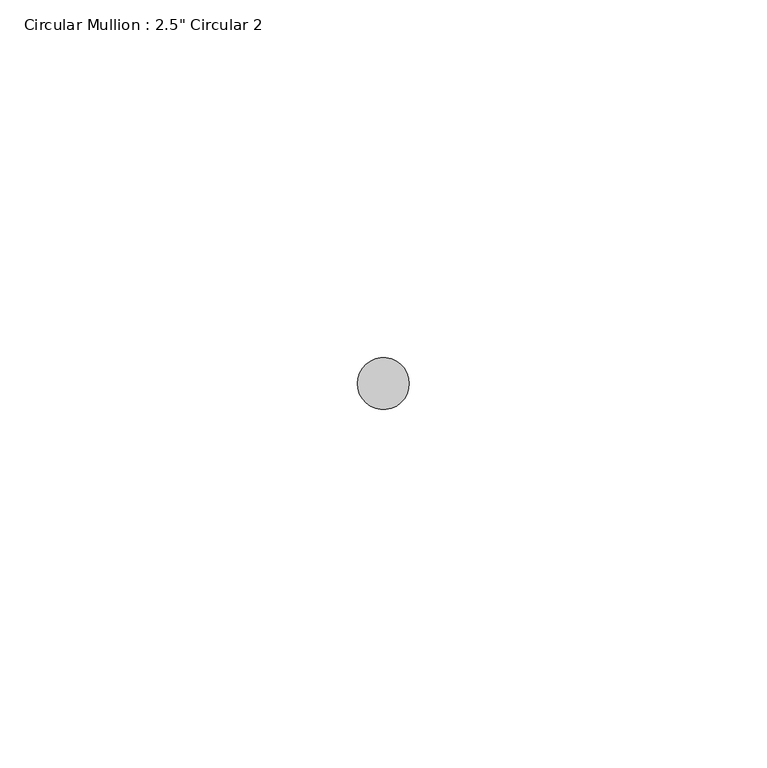
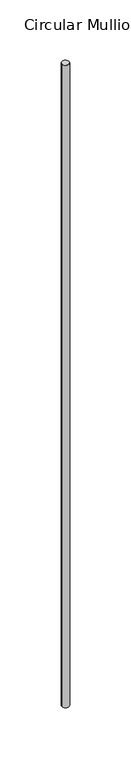
"""IFC4 building model written with IfcOpenShell, lengths in millimetres: member geometry."""

from ifc_helpers import new_model, si_unit, point, frame, frame_2d, origin, place, context, project, spatial, circle_curve, trimmed, segment, composite_curve, outline, extrude, source, transform, mapped, element, save


def member_e1a7572e(model_context):
    return source(origin(), model_context, "Body", "SweptSolid", [
        extrude(outline(composite_curve([segment(trimmed(circle_curve(frame_2d((-3.6195, 0.0)), 3.6195), [point((0.0, 0.0))], [point((-7.239, 0.0))], False, "CARTESIAN"), True, "CONTINUOUS"), segment(trimmed(circle_curve(frame_2d((-3.6195, 0.0)), 3.6195), [point((-7.239, 0.0))], [point((0.0, 0.0))], False, "CARTESIAN"), True, "CONTINUOUS")], self_intersect=False)), frame((0.0, 0.0, -659.511), z_axis=(0.0, 0.0, 1.0), x_axis=(1.0, 0.0, 0.0)), (0.0, 0.0, 1.0), 659.511),
    ])


if __name__ == "__main__":
    model = new_model("IFC4")
    model_context = context("Model", 3, world=origin())
    ifc_project = project(units=[si_unit("LENGTHUNIT", "METRE", prefix="MILLI")], contexts=[model_context])
    site = spatial("IfcSite", under=ifc_project)
    building = spatial("IfcBuilding", under=site)
    placement = place(None, origin())
    member_shape = member_e1a7572e(model_context)
    element("IfcMember", 1, ObjectType="Circular Mullion : 2.5\" Circular 2", at=placement, inside=building, context=model_context, shape_type="MappedRepresentation", body=[
        mapped(member_shape, transform((0.0, 0.0, 0.0), x_axis=(1.0, 0.0, 0.0), y_axis=(0.0, 1.0, 0.0), z_axis=(0.0, 0.0, 1.0))),
    ])
    save(model, "model.ifc")

# Revit data of these elements
# Type "Circular Mullion : 2.5\" Circular 2"
#   built-in parameter 1007350 = 0.011875 (stored number, unit not read)
# Element 1 (IfcMember, "Circular Mullion : 2.5\" Circular 2")
#   Materials on its faces: "Aluminum"
# Materials
#   "Aluminum": class "Metal", colour RGB 247 247 247, transparency 0, Description = "Aluminum 6061", Cost = 0
